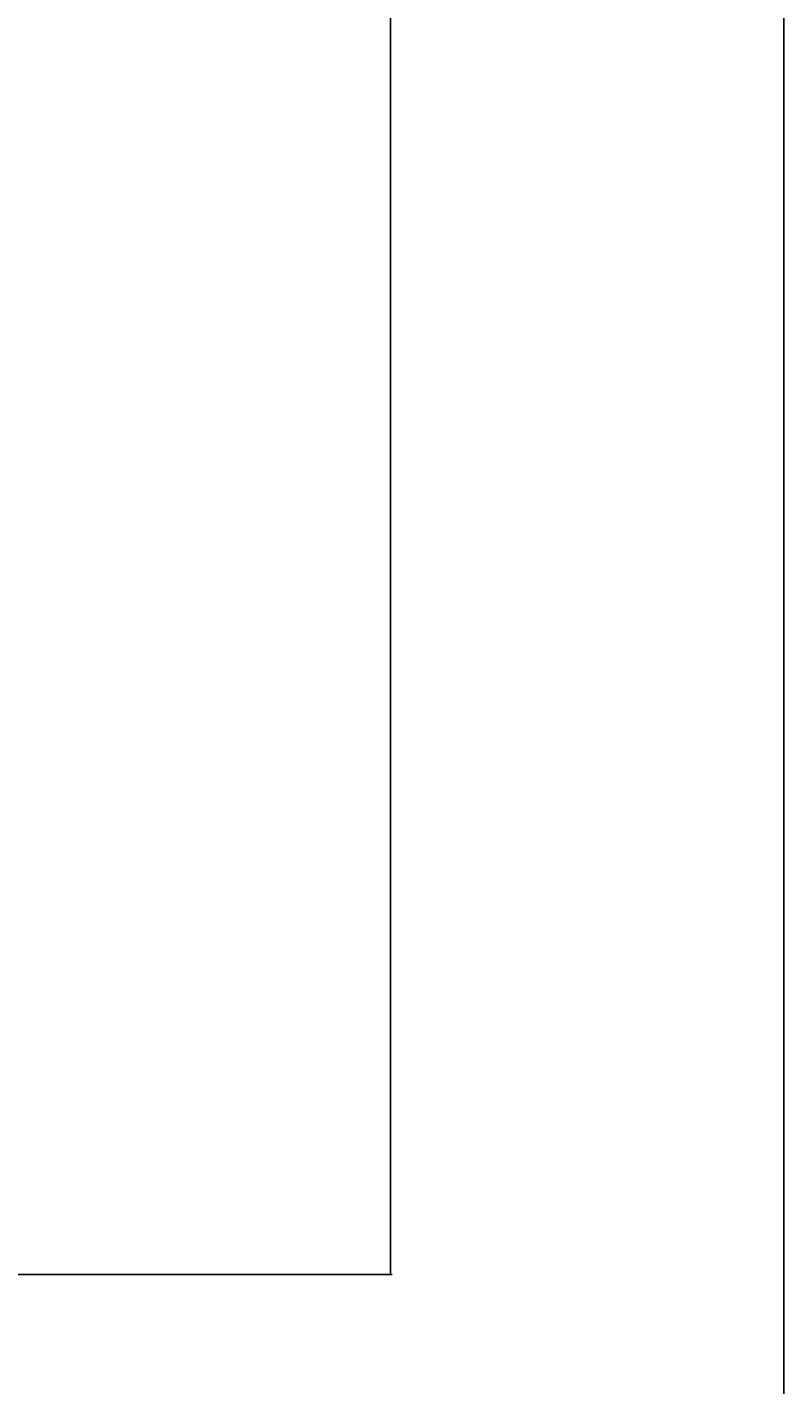
# Model space of a CAD drawing. Units: inches. Extents: x 1748 to 2382, y 1346 to 2284.
# Tile 15 of 26: x 2300 to 2382, y 1456 to 1604. Entities that reach past the tile are written whole.
import ezdxf

# ---------------------------------------------------------------- set-up
doc = ezdxf.new("R2010")
doc.units = ezdxf.units.IN
doc.layers.add('A-ANNO-DIMS', color=2, linetype='Continuous', lineweight=18)
doc.layers.add('A-ANNO-TTLB', color=7, linetype='Continuous', lineweight=25)
doc.styles.get("Standard").update_dxf_attribs({"font": 'arial.ttf'})
doc.dimstyles.get("Standard").update_dxf_attribs({"dimtxt": 0.18, "dimasz": 0.18, "dimexe": 0.18, "dimexo": 0.0625, "dimgap": 0.09, "dimtad": 0, "dimtih": 1, "dimtoh": 1, "dimdec": 4, "dimzin": 0, "dimdsep": 46, "dimtxsty": 'Standard', "dimcen": 0.09, "dimadec": 0, "dimazin": 0, "dimtfac": 1, "dimtdec": 4, "dimtofl": 0, "dimtmove": 0, "dimatfit": 3, "dimfxl": 1, "dimtolj": 1, "dimtzin": 0, "dimarcsym": 0})

# ---------------------------------------------------------------- blocks, each defined once
blk = doc.blocks.new('*D35')
at = {"layer": 'A-ANNO-DIMS', "color": 0, "lineweight": -2, "transparency": 16777216}
for p, q in [((2297.52, 2232.85), (2339.54, 2232.85)), ((2339.36, 2232.67), (2339.36, 1850.53)), ((2339.36, 1468.03), (2339.36, 1850.17)), ((2297.52, 1467.85), (2339.54, 1467.85))]:
    blk.add_line(p, q, dxfattribs=at)
at = {"layer": 'A-ANNO-DIMS', "color": 0, "transparency": 16777216}
for points in [[(2339.33, 2232.67), (2339.39, 2232.67), (2339.36, 2232.85)], [(2339.33, 1468.03), (2339.39, 1468.03), (2339.36, 1467.85)]]:
    blk.add_solid(points, dxfattribs=at)
at = {"layer": 'Defpoints', "color": 0, "transparency": 16777216}
for p in [(2297.46, 2232.85), (2339.36, 2232.85), (2297.46, 1467.85)]:
    blk.add_point(p, dxfattribs=at)
at = {"layer": 'A-ANNO-DIMS', "color": 0, "transparency": 16777216, "insert": (2339.36, 1850.35), "char_height": 0.18, "attachment_point": 5}
blk.add_mtext('\\A1;765', dxfattribs=at)

msp = doc.modelspace()

# ---------------------------------------------------------------- linework, layer by layer
at = {"layer": 'A-ANNO-TTLB'}
msp.add_lwpolyline([(1747.8112, 2284.3704), (2382.1361, 2284.3704), (2382.1361, 1346.4899), (1747.8112, 1346.4899)], close=True, dxfattribs=at)

# ---------------------------------------------------------------- dimensions: what is measured, and where the dimension line sits
at = {"layer": 'A-ANNO-DIMS'}
dim = msp.add_linear_dim(base=(2339.3607, 2232.8497), p1=(2297.4607, 1467.8497), p2=(2297.4607, 2232.8497), angle=90, dimstyle='Standard', override={"dimdec": 0, "dimlfac": 1, "dimrnd": 0, "dimzin": 0, "dimdsep": 46, "dimlunit": 2}, dxfattribs=at)
dim.commit()
dim.dimension.update_dxf_attribs({"geometry": '*D35', "text_midpoint": (2339.3607, 1850.3497)})

doc.saveas('drawing.dxf')
